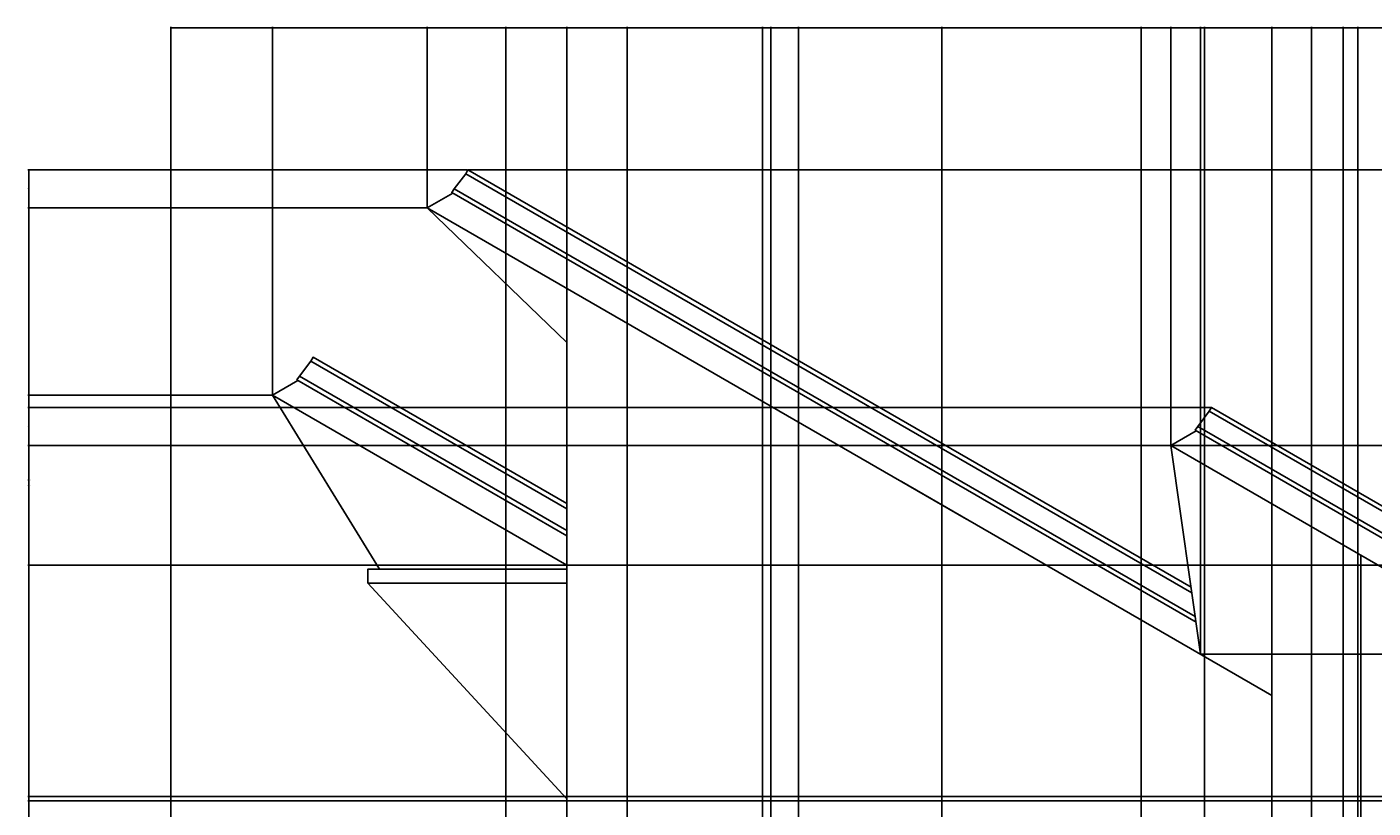
# Model space of a CAD drawing. Units: millimetres. Extents: x 171 to 1599, y 973 to 1509.
# Tile 4 of 7: x 951 to 1235, y 1343 to 1508. Entities that reach past the tile are written whole.
import ezdxf

# ---------------------------------------------------------------- set-up
doc = ezdxf.new("R2010")
doc.units = ezdxf.units.MM
doc.layers.add('A-ANNO-DIMS', color=2, linetype='Continuous', lineweight=18)
doc.layers.add('A-ELEV', color=7, linetype='Continuous', lineweight=25)
doc.styles.get("Standard").update_dxf_attribs({"font": 'arial.ttf'})
doc.dimstyles.get("Standard").update_dxf_attribs({"dimtxt": 0.18, "dimasz": 0.18, "dimexe": 0.18, "dimexo": 0.0625, "dimgap": 0.09, "dimtad": 0, "dimtih": 1, "dimtoh": 1, "dimdec": 1, "dimzin": 0, "dimdsep": 46, "dimlunit": 3, "dimtxsty": 'Standard', "dimcen": 0.09, "dimadec": 0, "dimazin": 0, "dimtfac": 1, "dimtdec": 1, "dimtofl": 0, "dimtmove": 0, "dimatfit": 3, "dimfxl": 1, "dimtolj": 1, "dimtzin": 0, "dimarcsym": 0})

# ---------------------------------------------------------------- blocks, each defined once
blk = doc.blocks.new('*D1')
at = {"layer": 'A-ANNO-DIMS', "color": 0, "lineweight": -2, "transparency": 16777216}
for p, q in [((980.93, 1194.55), (980.93, 1508.31)), ((981.11, 1508.13), (1274.61, 1508.13)), ((1568.85, 1508.13), (1275.36, 1508.13)), ((1569.03, 1215.31), (1569.03, 1508.31))]:
    blk.add_line(p, q, dxfattribs=at)
at = {"layer": 'A-ANNO-DIMS', "color": 0, "transparency": 16777216}
for points in [[(981.11, 1508.16), (981.11, 1508.1), (980.93, 1508.13)], [(1568.85, 1508.16), (1568.85, 1508.1), (1569.03, 1508.13)]]:
    blk.add_solid(points, dxfattribs=at)
at = {"layer": 'Defpoints', "color": 0, "transparency": 16777216}
for p in [(1569.03, 1508.13), (1569.03, 1215.25), (980.93, 1194.49)]:
    blk.add_point(p, dxfattribs=at)
at = {"layer": 'A-ANNO-DIMS', "color": 0, "transparency": 16777216, "insert": (1274.98, 1508.13), "char_height": 0.18, "attachment_point": 5}
blk.add_mtext('\\A1;588.1', dxfattribs=at)
blk = doc.blocks.new('*D2')
at = {"layer": 'A-ANNO-DIMS', "color": 0, "lineweight": -2, "transparency": 16777216}
for p, q in [((1043.70287, 1478.130098), (1599.212656, 1478.130098)), ((1599.032656, 1477.950098), (1599.032656, 1240.959874)), ((1599.032656, 1003.60965), (1599.032656, 1240.599874)), ((1348.449149, 1003.42965), (1599.212656, 1003.42965))]:
    blk.add_line(p, q, dxfattribs=at)
at = {"layer": 'A-ANNO-DIMS', "color": 0, "transparency": 16777216}
for points in [[(1599.002656, 1477.950098), (1599.062656, 1477.950098), (1599.032656, 1478.130098)], [(1599.002656, 1003.60965), (1599.062656, 1003.60965), (1599.032656, 1003.42965)]]:
    blk.add_solid(points, dxfattribs=at)
at = {"layer": 'Defpoints', "color": 0, "transparency": 16777216}
for p in [(1043.64037, 1478.130098), (1599.032656, 1478.130098), (1348.386649, 1003.42965)]:
    blk.add_point(p, dxfattribs=at)
at = {"layer": 'A-ANNO-DIMS', "color": 0, "transparency": 16777216, "insert": (1599.032656, 1240.779874), "char_height": 0.18, "attachment_point": 5}
blk.add_mtext('\\A1;474.7', dxfattribs=at)
blk = doc.blocks.new('*D17')
at = {"layer": 'A-ANNO-DIMS', "color": 0, "lineweight": -2, "transparency": 16777216}
for p, q in [((1105.76, 1344.87), (950.75, 1344.87)), ((950.93, 1344.69), (950.93, 1281.55)), ((950.93, 1218.05), (950.93, 1281.19)), ((1105.76, 1217.87), (950.75, 1217.87))]:
    blk.add_line(p, q, dxfattribs=at)
at = {"layer": 'A-ANNO-DIMS', "color": 0, "transparency": 16777216}
for points in [[(950.9, 1344.69), (950.96, 1344.69), (950.93, 1344.87)], [(950.9, 1218.05), (950.96, 1218.05), (950.93, 1217.87)]]:
    blk.add_solid(points, dxfattribs=at)
at = {"layer": 'Defpoints', "color": 0, "transparency": 16777216}
for p in [(950.93, 1344.87), (1105.82, 1344.87), (1105.82, 1217.87)]:
    blk.add_point(p, dxfattribs=at)
at = {"layer": 'A-ANNO-DIMS', "color": 0, "transparency": 16777216, "insert": (950.93, 1281.37), "char_height": 0.18, "attachment_point": 5}
blk.add_mtext('\\A1;127', dxfattribs=at)
blk = doc.blocks.new('*D18')
at = {"layer": 'A-ANNO-DIMS', "color": 0, "lineweight": -2, "transparency": 16777216}
for p, q in [((1043.58, 1478.13), (950.75, 1478.13)), ((950.93, 1477.95), (950.93, 1411.68)), ((950.93, 1345.05), (950.93, 1411.32)), ((1105.76, 1344.87), (950.75, 1344.87))]:
    blk.add_line(p, q, dxfattribs=at)
at = {"layer": 'A-ANNO-DIMS', "color": 0, "transparency": 16777216}
for points in [[(950.9, 1477.95), (950.96, 1477.95), (950.93, 1478.13)], [(950.9, 1345.05), (950.96, 1345.05), (950.93, 1344.87)]]:
    blk.add_solid(points, dxfattribs=at)
at = {"layer": 'Defpoints', "color": 0, "transparency": 16777216}
for p in [(950.93, 1478.13), (1043.64, 1478.13), (1105.82, 1344.87)]:
    blk.add_point(p, dxfattribs=at)
at = {"layer": 'A-ANNO-DIMS', "color": 0, "transparency": 16777216, "insert": (950.93, 1411.5), "char_height": 0.18, "attachment_point": 5}
blk.add_mtext('\\A1;133.26', dxfattribs=at)
blk = doc.blocks.new('*D38')
at = {"layer": 'A-ANNO-DIMS', "color": 0, "lineweight": -2, "transparency": 16777216}
for p, q in [((980.93, 1203.86), (980.93, 1508.31)), ((981.11, 1508.13), (991.19, 1508.13)), ((1002.21, 1508.13), (992.12, 1508.13)), ((1002.39, 1430.6), (1002.39, 1508.31))]:
    blk.add_line(p, q, dxfattribs=at)
at = {"layer": 'A-ANNO-DIMS', "color": 0, "transparency": 16777216}
for points in [[(981.11, 1508.16), (981.11, 1508.1), (980.93, 1508.13)], [(1002.21, 1508.16), (1002.21, 1508.1), (1002.39, 1508.13)]]:
    blk.add_solid(points, dxfattribs=at)
at = {"layer": 'Defpoints', "color": 0, "transparency": 16777216}
for p in [(1002.39, 1508.13), (1002.39, 1430.53), (980.93, 1203.79)]:
    blk.add_point(p, dxfattribs=at)
at = {"layer": 'A-ANNO-DIMS', "color": 0, "transparency": 16777216, "insert": (991.66, 1508.13), "char_height": 0.18, "attachment_point": 5}
blk.add_mtext('\\A1;21.455', dxfattribs=at)
blk = doc.blocks.new('*D39')
at = {"layer": 'A-ANNO-DIMS', "color": 0, "lineweight": -2, "transparency": 16777216}
for p, q in [((1002.39, 1430.6), (1002.39, 1508.31)), ((1002.57, 1508.13), (1033.05, 1508.13)), ((1064.32, 1508.13), (1033.84, 1508.13)), ((1064.5, 1394.73), (1064.5, 1508.31))]:
    blk.add_line(p, q, dxfattribs=at)
at = {"layer": 'A-ANNO-DIMS', "color": 0, "transparency": 16777216}
for points in [[(1002.57, 1508.16), (1002.57, 1508.1), (1002.39, 1508.13)], [(1064.32, 1508.16), (1064.32, 1508.1), (1064.5, 1508.13)]]:
    blk.add_solid(points, dxfattribs=at)
at = {"layer": 'Defpoints', "color": 0, "transparency": 16777216}
for p in [(1064.5, 1508.13), (1002.39, 1430.53), (1064.5, 1394.67)]:
    blk.add_point(p, dxfattribs=at)
at = {"layer": 'A-ANNO-DIMS', "color": 0, "transparency": 16777216, "insert": (1033.45, 1508.13), "char_height": 0.18, "attachment_point": 5}
blk.add_mtext('\\A1;62.12', dxfattribs=at)
blk = doc.blocks.new('*D40')
at = {"layer": 'A-ANNO-DIMS', "color": 0, "lineweight": -2, "transparency": 16777216}
for p, q in [((1002.39, 1430.6), (1002.39, 1508.31)), ((1002.57, 1508.13), (1018.33, 1508.13)), ((1034.88, 1508.13), (1019.12, 1508.13)), ((1035.06, 1470.15), (1035.06, 1508.31))]:
    blk.add_line(p, q, dxfattribs=at)
at = {"layer": 'A-ANNO-DIMS', "color": 0, "transparency": 16777216}
for points in [[(1002.57, 1508.16), (1002.57, 1508.1), (1002.39, 1508.13)], [(1034.88, 1508.16), (1034.88, 1508.1), (1035.06, 1508.13)]]:
    blk.add_solid(points, dxfattribs=at)
at = {"layer": 'Defpoints', "color": 0, "transparency": 16777216}
for p in [(1035.06, 1508.13), (1035.06, 1470.09), (1002.39, 1430.53)]:
    blk.add_point(p, dxfattribs=at)
at = {"layer": 'A-ANNO-DIMS', "color": 0, "transparency": 16777216, "insert": (1018.72, 1508.13), "char_height": 0.18, "attachment_point": 5}
blk.add_mtext('\\A1;32.68', dxfattribs=at)
blk = doc.blocks.new('*D41')
at = {"layer": 'A-ANNO-DIMS', "color": 0, "lineweight": -2, "transparency": 16777216}
for p, q in [((1035.06, 1470.15), (1035.06, 1508.31)), ((1035.24, 1508.13), (1116.22, 1508.13)), ((1198.11, 1508.13), (1117.13, 1508.13)), ((1198.29, 1375.91), (1198.29, 1508.31))]:
    blk.add_line(p, q, dxfattribs=at)
at = {"layer": 'A-ANNO-DIMS', "color": 0, "transparency": 16777216}
for points in [[(1035.24, 1508.16), (1035.24, 1508.1), (1035.06, 1508.13)], [(1198.11, 1508.16), (1198.11, 1508.1), (1198.29, 1508.13)]]:
    blk.add_solid(points, dxfattribs=at)
at = {"layer": 'Defpoints', "color": 0, "transparency": 16777216}
for p in [(1198.29, 1508.13), (1035.06, 1470.09), (1198.29, 1375.85)]:
    blk.add_point(p, dxfattribs=at)
at = {"layer": 'A-ANNO-DIMS', "color": 0, "transparency": 16777216, "insert": (1116.68, 1508.13), "char_height": 0.18, "attachment_point": 5}
blk.add_mtext('\\A1;163.23', dxfattribs=at)
blk = doc.blocks.new('*D42')
at = {"layer": 'A-ANNO-DIMS', "color": 0, "lineweight": -2, "transparency": 16777216}
for p, q in [((1192.02, 1419.99), (1192.02, 1508.31)), ((1192.2, 1508.13), (1378.72, 1508.13)), ((1566.18, 1508.13), (1379.65, 1508.13)), ((1566.36, 1203.87), (1566.36, 1508.31))]:
    blk.add_line(p, q, dxfattribs=at)
at = {"layer": 'A-ANNO-DIMS', "color": 0, "transparency": 16777216}
for points in [[(1192.2, 1508.16), (1192.2, 1508.1), (1192.02, 1508.13)], [(1566.18, 1508.16), (1566.18, 1508.1), (1566.36, 1508.13)]]:
    blk.add_solid(points, dxfattribs=at)
at = {"layer": 'Defpoints', "color": 0, "transparency": 16777216}
for p in [(1566.36, 1508.13), (1192.02, 1419.93), (1566.36, 1203.8)]:
    blk.add_point(p, dxfattribs=at)
at = {"layer": 'A-ANNO-DIMS', "color": 0, "transparency": 16777216, "insert": (1379.19, 1508.13), "char_height": 0.18, "attachment_point": 5}
blk.add_mtext('\\A1;374.34', dxfattribs=at)
blk = doc.blocks.new('*D43')
at = {"layer": 'A-ANNO-DIMS', "color": 0, "lineweight": -2, "transparency": 16777216}
for p, q in [((1002.32, 1430.53), (950.75, 1430.53)), ((950.93, 1430.35), (950.93, 1412.78)), ((950.93, 1394.85), (950.93, 1412.42)), ((1064.44, 1394.67), (950.75, 1394.67))]:
    blk.add_line(p, q, dxfattribs=at)
at = {"layer": 'A-ANNO-DIMS', "color": 0, "transparency": 16777216}
for points in [[(950.9, 1430.35), (950.96, 1430.35), (950.93, 1430.53)], [(950.9, 1394.85), (950.96, 1394.85), (950.93, 1394.67)]]:
    blk.add_solid(points, dxfattribs=at)
at = {"layer": 'Defpoints', "color": 0, "transparency": 16777216}
for p in [(1002.39, 1430.53), (950.93, 1394.67), (1064.5, 1394.67)]:
    blk.add_point(p, dxfattribs=at)
at = {"layer": 'A-ANNO-DIMS', "color": 0, "transparency": 16777216, "insert": (950.93, 1412.6), "char_height": 0.18, "attachment_point": 5}
blk.add_mtext('\\A1;35.865', dxfattribs=at)
blk = doc.blocks.new('*D44')
at = {"layer": 'A-ANNO-DIMS', "color": 0, "lineweight": -2, "transparency": 16777216}
for p, q in [((1043.58, 1478.13), (950.75, 1478.13)), ((950.93, 1477.95), (950.93, 1474.29)), ((950.93, 1470.27), (950.93, 1473.93)), ((1035, 1470.09), (950.75, 1470.09))]:
    blk.add_line(p, q, dxfattribs=at)
at = {"layer": 'A-ANNO-DIMS', "color": 0, "transparency": 16777216}
for points in [[(950.9, 1477.95), (950.96, 1477.95), (950.93, 1478.13)], [(950.9, 1470.27), (950.96, 1470.27), (950.93, 1470.09)]]:
    blk.add_solid(points, dxfattribs=at)
at = {"layer": 'Defpoints', "color": 0, "transparency": 16777216}
for p in [(950.93, 1478.13), (1043.64, 1478.13), (1035.06, 1470.09)]:
    blk.add_point(p, dxfattribs=at)
at = {"layer": 'A-ANNO-DIMS', "color": 0, "transparency": 16777216, "insert": (950.93, 1474.11), "char_height": 0.18, "attachment_point": 5}
blk.add_mtext('\\A1;8.04', dxfattribs=at)
blk = doc.blocks.new('*D45')
at = {"layer": 'A-ANNO-DIMS', "color": 0, "lineweight": -2, "transparency": 16777216}
for p, q in [((1064.57, 1394.67), (1599.21, 1394.67)), ((1599.03, 1394.49), (1599.03, 1369.95)), ((1599.03, 1345.05), (1599.03, 1369.59)), ((1105.88, 1344.87), (1599.21, 1344.87))]:
    blk.add_line(p, q, dxfattribs=at)
at = {"layer": 'A-ANNO-DIMS', "color": 0, "transparency": 16777216}
for points in [[(1599, 1394.49), (1599.06, 1394.49), (1599.03, 1394.67)], [(1599, 1345.05), (1599.06, 1345.05), (1599.03, 1344.87)]]:
    blk.add_solid(points, dxfattribs=at)
at = {"layer": 'Defpoints', "color": 0, "transparency": 16777216}
for p in [(1064.5, 1394.67), (1105.82, 1344.87), (1599.03, 1344.87)]:
    blk.add_point(p, dxfattribs=at)
at = {"layer": 'A-ANNO-DIMS', "color": 0, "transparency": 16777216, "insert": (1599.03, 1369.77), "char_height": 0.18, "attachment_point": 5}
blk.add_mtext('\\A1;49.80', dxfattribs=at)
blk = doc.blocks.new('*D46')
at = {"layer": 'A-ANNO-DIMS', "color": 0, "lineweight": -2, "transparency": 16777216}
for p, q in [((1198.36, 1375.85), (1599.21, 1375.85)), ((1599.03, 1375.67), (1599.03, 1360.54)), ((1599.03, 1345.05), (1599.03, 1360.18)), ((1185.8, 1344.87), (1599.21, 1344.87))]:
    blk.add_line(p, q, dxfattribs=at)
at = {"layer": 'A-ANNO-DIMS', "color": 0, "transparency": 16777216}
for points in [[(1599, 1375.67), (1599.06, 1375.67), (1599.03, 1375.85)], [(1599, 1345.05), (1599.06, 1345.05), (1599.03, 1344.87)]]:
    blk.add_solid(points, dxfattribs=at)
at = {"layer": 'Defpoints', "color": 0, "transparency": 16777216}
for p in [(1198.29, 1375.85), (1599.03, 1375.85), (1185.73, 1344.87)]:
    blk.add_point(p, dxfattribs=at)
at = {"layer": 'A-ANNO-DIMS', "color": 0, "transparency": 16777216, "insert": (1599.03, 1360.36), "char_height": 0.18, "attachment_point": 5}
blk.add_mtext('\\A1;30.976', dxfattribs=at)
blk = doc.blocks.new('*D47')
at = {"layer": 'A-ANNO-DIMS', "color": 0, "lineweight": -2, "transparency": 16777216}
for p, q in [((1192.08, 1419.93), (1599.21, 1419.93)), ((1599.03, 1419.75), (1599.03, 1312.05)), ((1599.03, 1203.98), (1599.03, 1311.68)), ((1566.42, 1203.8), (1599.21, 1203.8))]:
    blk.add_line(p, q, dxfattribs=at)
at = {"layer": 'A-ANNO-DIMS', "color": 0, "transparency": 16777216}
for points in [[(1599, 1419.75), (1599.06, 1419.75), (1599.03, 1419.93)], [(1599, 1203.98), (1599.06, 1203.98), (1599.03, 1203.8)]]:
    blk.add_solid(points, dxfattribs=at)
at = {"layer": 'Defpoints', "color": 0, "transparency": 16777216}
for p in [(1192.02, 1419.93), (1566.36, 1203.8), (1599.03, 1203.8)]:
    blk.add_point(p, dxfattribs=at)
at = {"layer": 'A-ANNO-DIMS', "color": 0, "transparency": 16777216, "insert": (1599.03, 1311.87), "char_height": 0.18, "attachment_point": 5}
blk.add_mtext('\\A1;216.13', dxfattribs=at)
blk = doc.blocks.new('*D48')
at = {"layer": 'A-ANNO-DIMS', "color": 0, "lineweight": -2, "transparency": 16777216}
for p, q in [((1200.53, 1427.97), (950.75, 1427.97)), ((950.93, 1427.79), (950.93, 1424.13)), ((950.93, 1420.11), (950.93, 1423.77)), ((1191.95, 1419.93), (950.75, 1419.93))]:
    blk.add_line(p, q, dxfattribs=at)
at = {"layer": 'A-ANNO-DIMS', "color": 0, "transparency": 16777216}
for points in [[(950.9, 1427.79), (950.96, 1427.79), (950.93, 1427.97)], [(950.9, 1420.11), (950.96, 1420.11), (950.93, 1419.93)]]:
    blk.add_solid(points, dxfattribs=at)
at = {"layer": 'Defpoints', "color": 0, "transparency": 16777216}
for p in [(950.93, 1427.97), (1200.59, 1427.97), (1192.02, 1419.93)]:
    blk.add_point(p, dxfattribs=at)
at = {"layer": 'A-ANNO-DIMS', "color": 0, "transparency": 16777216, "insert": (950.93, 1423.95), "char_height": 0.18, "attachment_point": 5}
blk.add_mtext('\\A1;8.04', dxfattribs=at)
blk = doc.blocks.new('*D49')
at = {"layer": 'A-ANNO-DIMS', "color": 0, "lineweight": -2, "transparency": 16777216}
for p, q in [((1064.5, 1203.86), (1064.5, 1508.31)), ((1064.68, 1508.13), (1084.78, 1508.13)), ((1105.64, 1508.13), (1085.54, 1508.13)), ((1105.82, 1344.93), (1105.82, 1508.31))]:
    blk.add_line(p, q, dxfattribs=at)
at = {"layer": 'A-ANNO-DIMS', "color": 0, "transparency": 16777216}
for points in [[(1064.68, 1508.16), (1064.68, 1508.1), (1064.5, 1508.13)], [(1105.64, 1508.16), (1105.64, 1508.1), (1105.82, 1508.13)]]:
    blk.add_solid(points, dxfattribs=at)
at = {"layer": 'Defpoints', "color": 0, "transparency": 16777216}
for p in [(1105.82, 1508.13), (1105.82, 1344.87), (1064.5, 1203.79)]:
    blk.add_point(p, dxfattribs=at)
at = {"layer": 'A-ANNO-DIMS', "color": 0, "transparency": 16777216, "insert": (1085.16, 1508.13), "char_height": 0.18, "attachment_point": 5}
blk.add_mtext('\\A1;41.31', dxfattribs=at)
blk = doc.blocks.new('*D50')
at = {"layer": 'A-ANNO-DIMS', "color": 0, "lineweight": -2, "transparency": 16777216}
for p, q in [((1105.82, 1344.93), (1105.82, 1508.31)), ((1106, 1508.13), (1145.38, 1508.13)), ((1185.55, 1508.13), (1146.17, 1508.13)), ((1185.73, 1344.93), (1185.73, 1508.31))]:
    blk.add_line(p, q, dxfattribs=at)
at = {"layer": 'A-ANNO-DIMS', "color": 0, "transparency": 16777216}
for points in [[(1106, 1508.16), (1106, 1508.1), (1105.82, 1508.13)], [(1185.55, 1508.16), (1185.55, 1508.1), (1185.73, 1508.13)]]:
    blk.add_solid(points, dxfattribs=at)
at = {"layer": 'Defpoints', "color": 0, "transparency": 16777216}
for p in [(1185.73, 1508.13), (1105.82, 1344.87), (1185.73, 1344.87)]:
    blk.add_point(p, dxfattribs=at)
at = {"layer": 'A-ANNO-DIMS', "color": 0, "transparency": 16777216, "insert": (1145.78, 1508.13), "char_height": 0.18, "attachment_point": 5}
blk.add_mtext('\\A1;79.92', dxfattribs=at)
blk = doc.blocks.new('*D51')
at = {"layer": 'A-ANNO-DIMS', "color": 0, "lineweight": -2, "transparency": 16777216}
for p, q in [((1185.73, 1344.93), (1185.73, 1508.31)), ((1185.91, 1508.13), (1199.08, 1508.13)), ((1213.17, 1508.13), (1200.01, 1508.13)), ((1213.35, 1203.86), (1213.35, 1508.31))]:
    blk.add_line(p, q, dxfattribs=at)
at = {"layer": 'A-ANNO-DIMS', "color": 0, "transparency": 16777216}
for points in [[(1185.91, 1508.16), (1185.91, 1508.1), (1185.73, 1508.13)], [(1213.17, 1508.16), (1213.17, 1508.1), (1213.35, 1508.13)]]:
    blk.add_solid(points, dxfattribs=at)
at = {"layer": 'Defpoints', "color": 0, "transparency": 16777216}
for p in [(1213.35, 1508.13), (1185.73, 1344.87), (1213.35, 1203.79)]:
    blk.add_point(p, dxfattribs=at)
at = {"layer": 'A-ANNO-DIMS', "color": 0, "transparency": 16777216, "insert": (1199.54, 1508.13), "char_height": 0.18, "attachment_point": 5}
blk.add_mtext('\\A1;27.614', dxfattribs=at)
blk = doc.blocks.new('*D61')
at = {"layer": 'A-ANNO-DIMS', "color": 0, "lineweight": -2, "transparency": 16777216}
for p, q in [((1320.26, 1345.85), (950.75, 1345.85)), ((950.93, 1345.67), (950.93, 1269.24)), ((950.93, 1192.45), (950.93, 1268.88)), ((1320.26, 1192.27), (950.75, 1192.27))]:
    blk.add_line(p, q, dxfattribs=at)
at = {"layer": 'A-ANNO-DIMS', "color": 0, "transparency": 16777216}
for points in [[(950.9, 1345.67), (950.96, 1345.67), (950.93, 1345.85)], [(950.9, 1192.45), (950.96, 1192.45), (950.93, 1192.27)]]:
    blk.add_solid(points, dxfattribs=at)
at = {"layer": 'Defpoints', "color": 0, "transparency": 16777216}
for p in [(950.93, 1345.85), (1320.32, 1345.85), (1320.32, 1192.27)]:
    blk.add_point(p, dxfattribs=at)
at = {"layer": 'A-ANNO-DIMS', "color": 0, "transparency": 16777216, "insert": (950.93, 1269.06), "char_height": 0.18, "attachment_point": 5}
blk.add_mtext('\\A1;153.59', dxfattribs=at)
blk = doc.blocks.new('*D64')
at = {"layer": 'A-ANNO-DIMS', "color": 0, "lineweight": -2, "transparency": 16777216}
for p, q in [((1051.62, 1177.93), (1051.62, 1508.31)), ((1051.8, 1508.13), (1057.61, 1508.13)), ((1064.32, 1508.13), (1058.52, 1508.13)), ((1064.5, 1177.93), (1064.5, 1508.31))]:
    blk.add_line(p, q, dxfattribs=at)
at = {"layer": 'A-ANNO-DIMS', "color": 0, "transparency": 16777216}
for points in [[(1051.8, 1508.16), (1051.8, 1508.1), (1051.62, 1508.13)], [(1064.32, 1508.16), (1064.32, 1508.1), (1064.5, 1508.13)]]:
    blk.add_solid(points, dxfattribs=at)
at = {"layer": 'Defpoints', "color": 0, "transparency": 16777216}
for p in [(1064.5, 1508.13), (1051.62, 1177.87), (1064.5, 1177.87)]:
    blk.add_point(p, dxfattribs=at)
at = {"layer": 'A-ANNO-DIMS', "color": 0, "transparency": 16777216, "insert": (1058.06, 1508.13), "char_height": 0.18, "attachment_point": 5}
blk.add_mtext('\\A1;12.882', dxfattribs=at)
blk = doc.blocks.new('*D65')
at = {"layer": 'A-ANNO-DIMS', "color": 0, "lineweight": -2, "transparency": 16777216}
for p, q in [((1064.5, 1177.93), (1064.5, 1508.31)), ((1064.68, 1508.13), (1070.43, 1508.13)), ((1077.09, 1508.13), (1071.34, 1508.13)), ((1077.27, 1177.93), (1077.27, 1508.31))]:
    blk.add_line(p, q, dxfattribs=at)
at = {"layer": 'A-ANNO-DIMS', "color": 0, "transparency": 16777216}
for points in [[(1064.68, 1508.16), (1064.68, 1508.1), (1064.5, 1508.13)], [(1077.09, 1508.16), (1077.09, 1508.1), (1077.27, 1508.13)]]:
    blk.add_solid(points, dxfattribs=at)
at = {"layer": 'Defpoints', "color": 0, "transparency": 16777216}
for p in [(1077.27, 1508.13), (1064.5, 1177.87), (1077.27, 1177.87)]:
    blk.add_point(p, dxfattribs=at)
at = {"layer": 'A-ANNO-DIMS', "color": 0, "transparency": 16777216, "insert": (1070.89, 1508.13), "char_height": 0.18, "attachment_point": 5}
blk.add_mtext('\\A1;12.767', dxfattribs=at)
blk = doc.blocks.new('*D66')
at = {"layer": 'A-ANNO-DIMS', "color": 0, "lineweight": -2, "transparency": 16777216}
for p, q in [((1077.27, 1177.93), (1077.27, 1508.31)), ((1077.45, 1508.13), (1092.02, 1508.13)), ((1107.38, 1508.13), (1092.81, 1508.13)), ((1107.56, 1177.93), (1107.56, 1508.31))]:
    blk.add_line(p, q, dxfattribs=at)
at = {"layer": 'A-ANNO-DIMS', "color": 0, "transparency": 16777216}
for points in [[(1077.45, 1508.16), (1077.45, 1508.1), (1077.27, 1508.13)], [(1107.38, 1508.16), (1107.38, 1508.1), (1107.56, 1508.13)]]:
    blk.add_solid(points, dxfattribs=at)
at = {"layer": 'Defpoints', "color": 0, "transparency": 16777216}
for p in [(1107.56, 1508.13), (1077.27, 1177.87), (1107.56, 1177.87)]:
    blk.add_point(p, dxfattribs=at)
at = {"layer": 'A-ANNO-DIMS', "color": 0, "transparency": 16777216, "insert": (1092.42, 1508.13), "char_height": 0.18, "attachment_point": 5}
blk.add_mtext('\\A1;30.29', dxfattribs=at)
blk = doc.blocks.new('*D67')
at = {"layer": 'A-ANNO-DIMS', "color": 0, "lineweight": -2, "transparency": 16777216}
for p, q in [((1107.56, 1177.93), (1107.56, 1508.31)), ((1107.74, 1508.13), (1110.09, 1508.13)), ((1113.23, 1508.13), (1110.88, 1508.13)), ((1113.41, 1177.93), (1113.41, 1508.31))]:
    blk.add_line(p, q, dxfattribs=at)
at = {"layer": 'A-ANNO-DIMS', "color": 0, "transparency": 16777216}
for points in [[(1107.74, 1508.16), (1107.74, 1508.1), (1107.56, 1508.13)], [(1113.23, 1508.16), (1113.23, 1508.1), (1113.41, 1508.13)]]:
    blk.add_solid(points, dxfattribs=at)
at = {"layer": 'Defpoints', "color": 0, "transparency": 16777216}
for p in [(1113.41, 1508.13), (1107.56, 1177.87), (1113.41, 1177.87)]:
    blk.add_point(p, dxfattribs=at)
at = {"layer": 'A-ANNO-DIMS', "color": 0, "transparency": 16777216, "insert": (1110.49, 1508.13), "char_height": 0.18, "attachment_point": 5}
blk.add_mtext('\\A1;5.847', dxfattribs=at)
blk = doc.blocks.new('*D68')
at = {"layer": 'A-ANNO-DIMS', "color": 0, "lineweight": -2, "transparency": 16777216}
for p, q in [((1113.41, 1177.93), (1113.41, 1508.31)), ((1113.59, 1508.13), (1128.16, 1508.13)), ((1143.52, 1508.13), (1128.95, 1508.13)), ((1143.7, 1177.93), (1143.7, 1508.31))]:
    blk.add_line(p, q, dxfattribs=at)
at = {"layer": 'A-ANNO-DIMS', "color": 0, "transparency": 16777216}
for points in [[(1113.59, 1508.16), (1113.59, 1508.1), (1113.41, 1508.13)], [(1143.52, 1508.16), (1143.52, 1508.1), (1143.7, 1508.13)]]:
    blk.add_solid(points, dxfattribs=at)
at = {"layer": 'Defpoints', "color": 0, "transparency": 16777216}
for p in [(1143.7, 1508.13), (1113.41, 1177.87), (1143.7, 1177.87)]:
    blk.add_point(p, dxfattribs=at)
at = {"layer": 'A-ANNO-DIMS', "color": 0, "transparency": 16777216, "insert": (1128.55, 1508.13), "char_height": 0.18, "attachment_point": 5}
blk.add_mtext('\\A1;30.29', dxfattribs=at)
blk = doc.blocks.new('*D69')
at = {"layer": 'A-ANNO-DIMS', "color": 0, "lineweight": -2, "transparency": 16777216}
for p, q in [((1143.7, 1177.93), (1143.7, 1508.31)), ((1143.88, 1508.13), (1171.03, 1508.13)), ((1198.93, 1508.13), (1171.78, 1508.13)), ((1199.11, 1177.93), (1199.11, 1508.31))]:
    blk.add_line(p, q, dxfattribs=at)
at = {"layer": 'A-ANNO-DIMS', "color": 0, "transparency": 16777216}
for points in [[(1143.88, 1508.16), (1143.88, 1508.1), (1143.7, 1508.13)], [(1198.93, 1508.16), (1198.93, 1508.1), (1199.11, 1508.13)]]:
    blk.add_solid(points, dxfattribs=at)
at = {"layer": 'Defpoints', "color": 0, "transparency": 16777216}
for p in [(1199.11, 1508.13), (1143.7, 1177.87), (1199.11, 1177.87)]:
    blk.add_point(p, dxfattribs=at)
at = {"layer": 'A-ANNO-DIMS', "color": 0, "transparency": 16777216, "insert": (1171.4, 1508.13), "char_height": 0.18, "attachment_point": 5}
blk.add_mtext('\\A1;55.41', dxfattribs=at)
blk = doc.blocks.new('*D70')
at = {"layer": 'A-ANNO-DIMS', "color": 0, "lineweight": -2, "transparency": 16777216}
for p, q in [((1199.11, 1177.93), (1199.11, 1508.31)), ((1199.29, 1508.13), (1210.04, 1508.13)), ((1221.54, 1508.13), (1210.79, 1508.13)), ((1221.72, 1177.93), (1221.72, 1508.31))]:
    blk.add_line(p, q, dxfattribs=at)
at = {"layer": 'A-ANNO-DIMS', "color": 0, "transparency": 16777216}
for points in [[(1199.29, 1508.16), (1199.29, 1508.1), (1199.11, 1508.13)], [(1221.54, 1508.16), (1221.54, 1508.1), (1221.72, 1508.13)]]:
    blk.add_solid(points, dxfattribs=at)
at = {"layer": 'Defpoints', "color": 0, "transparency": 16777216}
for p in [(1221.72, 1508.13), (1199.11, 1177.87), (1221.72, 1177.87)]:
    blk.add_point(p, dxfattribs=at)
at = {"layer": 'A-ANNO-DIMS', "color": 0, "transparency": 16777216, "insert": (1210.41, 1508.13), "char_height": 0.18, "attachment_point": 5}
blk.add_mtext('\\A1;22.61', dxfattribs=at)
blk = doc.blocks.new('*D71')
at = {"layer": 'A-ANNO-DIMS', "color": 0, "lineweight": -2, "transparency": 16777216}
for p, q in [((1221.72, 1177.93), (1221.72, 1508.31)), ((1221.9, 1508.13), (1224.73, 1508.13)), ((1228.22, 1508.13), (1225.38, 1508.13)), ((1228.4, 1114.32), (1228.4, 1508.31))]:
    blk.add_line(p, q, dxfattribs=at)
at = {"layer": 'A-ANNO-DIMS', "color": 0, "transparency": 16777216}
for points in [[(1221.9, 1508.16), (1221.9, 1508.1), (1221.72, 1508.13)], [(1228.22, 1508.16), (1228.22, 1508.1), (1228.4, 1508.13)]]:
    blk.add_solid(points, dxfattribs=at)
at = {"layer": 'Defpoints', "color": 0, "transparency": 16777216}
for p in [(1228.4, 1508.13), (1221.72, 1177.87), (1228.4, 1114.25)]:
    blk.add_point(p, dxfattribs=at)
at = {"layer": 'A-ANNO-DIMS', "color": 0, "transparency": 16777216, "insert": (1225.06, 1508.13), "char_height": 0.18, "attachment_point": 5}
blk.add_mtext('\\A1;6.68', dxfattribs=at)
blk = doc.blocks.new('*D72')
at = {"layer": 'A-ANNO-DIMS', "color": 0, "lineweight": -2, "transparency": 16777216}
for p, q in [((1228.4, 1114.32), (1228.4, 1508.31)), ((1228.58, 1508.13), (1229.61, 1508.13)), ((1231.28, 1508.13), (1230.25, 1508.13)), ((1231.46, 1114.32), (1231.46, 1508.31))]:
    blk.add_line(p, q, dxfattribs=at)
at = {"layer": 'A-ANNO-DIMS', "color": 0, "transparency": 16777216}
for points in [[(1228.58, 1508.16), (1228.58, 1508.1), (1228.4, 1508.13)], [(1231.28, 1508.16), (1231.28, 1508.1), (1231.46, 1508.13)]]:
    blk.add_solid(points, dxfattribs=at)
at = {"layer": 'Defpoints', "color": 0, "transparency": 16777216}
for p in [(1231.46, 1508.13), (1228.4, 1114.25), (1231.46, 1114.25)]:
    blk.add_point(p, dxfattribs=at)
at = {"layer": 'A-ANNO-DIMS', "color": 0, "transparency": 16777216, "insert": (1229.93, 1508.13), "char_height": 0.18, "attachment_point": 5}
blk.add_mtext('\\A1;3.06', dxfattribs=at)
blk = doc.blocks.new('*D73')
at = {"layer": 'A-ANNO-DIMS', "color": 0, "lineweight": -2, "transparency": 16777216}
for p, q in [((1231.46, 1114.32), (1231.46, 1508.31)), ((1231.64, 1508.13), (1234.06, 1508.13)), ((1237.13, 1508.13), (1234.71, 1508.13)), ((1237.31, 1162.35), (1237.31, 1508.31))]:
    blk.add_line(p, q, dxfattribs=at)
at = {"layer": 'A-ANNO-DIMS', "color": 0, "transparency": 16777216}
for points in [[(1231.64, 1508.16), (1231.64, 1508.1), (1231.46, 1508.13)], [(1237.13, 1508.16), (1237.13, 1508.1), (1237.31, 1508.13)]]:
    blk.add_solid(points, dxfattribs=at)
at = {"layer": 'Defpoints', "color": 0, "transparency": 16777216}
for p in [(1237.31, 1508.13), (1237.31, 1162.29), (1231.46, 1114.25)]:
    blk.add_point(p, dxfattribs=at)
at = {"layer": 'A-ANNO-DIMS', "color": 0, "transparency": 16777216, "insert": (1234.38, 1508.13), "char_height": 0.18, "attachment_point": 5}
blk.add_mtext('\\A1;5.85', dxfattribs=at)

msp = doc.modelspace()

# ---------------------------------------------------------------- linework, layer by layer
at = {"layer": 'A-ELEV'}
for p, q in [((1043.1682, 1477.3124), (1196.447, 1388.8168)), ((1040.7486, 1474.1058), (1197.1614, 1383.8008)), ((1148.9051, 1404.3628), (1035.0626, 1470.0898)), ((1064.505, 1203.7941), (1064.505, 1453.0912)), ((1010.4912, 1437.7559), (1064.505, 1406.5711)), ((1007.5452, 1433.7629), (1064.505, 1400.8772)), ((1064.505, 1394.6687), (1002.3855, 1430.5334)), ((1197.176, 1423.1592), (1197.7023, 1423.9457)), ((1192.0162, 1419.9297), (1198.2939, 1375.8481)), ((1135.1656, 1412.2952), (1213.3488, 1367.1562)), ((1213.3488, 1203.7941), (1213.3488, 1407.6133)), ((1022.4961, 1390.8634), (1064.505, 1345.3593))]:
    msp.add_line(p, q, dxfattribs=at)
for points in [[(1040.2223, 1473.3193), (1040.7486, 1474.1058), (1043.1682, 1477.3124), (1043.6404, 1478.1301), (1196.2778, 1390.0048)], [(1197.3305, 1382.6128), (1040.2223, 1473.3193), (1040.4393, 1473.194), (1035.0626, 1470.0898), (1064.505, 1441.6631)], [(1008.0715, 1434.5494), (1010.4912, 1437.7559), (1010.9633, 1438.5737), (1064.505, 1407.6614)], [(1064.505, 1401.9675), (1008.0715, 1434.5494), (1007.5452, 1433.7629), (1007.7622, 1433.6376), (1002.3855, 1430.5334), (1024.973, 1393.7984)], [(1200.1219, 1427.1523), (1200.594, 1427.97), (1569.0327, 1215.2519), (1568.5605, 1214.4341), (1566.9934, 1210.7354), (1566.5754, 1209.8864), (1197.176, 1423.1592), (1197.3929, 1423.034), (1192.0162, 1419.9297), (1305.8587, 1354.2027), (1566.3585, 1203.8031), (1566.3585, 1210.0116)], [(1566.9934, 1210.7354), (1197.7023, 1423.9457), (1200.1219, 1427.1523), (1568.5605, 1214.4341)], [(1232.0993, 1203.7941), (1232.0993, 1396.7877)]]:
    msp.add_lwpolyline(points, dxfattribs=at)
for points in [[(1064.505, 1390.8634), (1022.4961, 1390.8634), (1022.4961, 1393.7984), (1064.505, 1393.7984)], [(1185.7346, 1217.867), (1105.8176, 1217.867), (1105.8176, 1344.8717), (1185.7346, 1344.8717)]]:
    msp.add_lwpolyline(points, close=True, dxfattribs=at)

# ---------------------------------------------------------------- dimensions: what is measured, and where the dimension line sits
at = {"layer": 'A-ANNO-DIMS'}
for base, p1, p2, override, picture, middle in [((1569.0327, 1508.1301), (980.9303, 1194.488), (1569.0327, 1215.2519), {"dimdec": 1, "dimlfac": 1, "dimrnd": 0, "dimzin": 0, "dimdsep": 46, "dimlunit": 2}, '*D1', (1274.9815, 1508.1301)), ((1002.3855, 1508.1301), (980.9303, 1203.7941), (1002.3855, 1430.5334), {"dimdec": 3, "dimlfac": 1, "dimrnd": 0, "dimzin": 0, "dimdsep": 46, "dimlunit": 2}, '*D38', (991.6579, 1508.1301)), ((1064.505, 1508.1301), (1002.3855, 1430.5334), (1064.505, 1394.6687), {"dimdec": 2, "dimlfac": 1, "dimrnd": 0, "dimzin": 0, "dimdsep": 46, "dimlunit": 2}, '*D39', (1033.4452, 1508.1301)), ((1035.0626, 1508.1301), (1002.3855, 1430.5334), (1035.0626, 1470.0898), {"dimdec": 2, "dimlfac": 1, "dimrnd": 0, "dimzin": 0, "dimdsep": 46, "dimlunit": 2}, '*D40', (1018.724, 1508.1301)), ((1198.2939, 1508.1301), (1035.0626, 1470.0898), (1198.2939, 1375.8481), {"dimdec": 2, "dimlfac": 1, "dimrnd": 0, "dimzin": 0, "dimdsep": 46, "dimlunit": 2}, '*D41', (1116.6782, 1508.1301)), ((1064.505, 1508.1301), (1051.6226, 1177.8722), (1064.505, 1177.8722), {"dimdec": 3, "dimlfac": 1, "dimrnd": 0, "dimzin": 0, "dimdsep": 46, "dimlunit": 2}, '*D64', (1058.0638, 1508.1301)), ((1105.8176, 1508.1301), (1064.505, 1203.7941), (1105.8176, 1344.8717), {"dimdec": 2, "dimlfac": 1, "dimrnd": 0, "dimzin": 0, "dimdsep": 46, "dimlunit": 2}, '*D49', (1085.1613, 1508.1301)), ((1077.2721, 1508.1301), (1064.505, 1177.8722), (1077.2721, 1177.8722), {"dimdec": 3, "dimlfac": 1, "dimrnd": 0, "dimzin": 0, "dimdsep": 46, "dimlunit": 2}, '*D65', (1070.8885, 1508.1301)), ((1107.5629, 1508.1301), (1077.2721, 1177.8722), (1107.5629, 1177.8722), {"dimdec": 2, "dimlfac": 1, "dimrnd": 0, "dimzin": 0, "dimdsep": 46, "dimlunit": 2}, '*D66', (1092.4175, 1508.1301)), ((1185.7346, 1508.1301), (1105.8176, 1344.8717), (1185.7346, 1344.8717), {"dimdec": 2, "dimlfac": 1, "dimrnd": 0, "dimzin": 0, "dimdsep": 46, "dimlunit": 2}, '*D50', (1145.7761, 1508.1301)), ((1113.4097, 1508.1301), (1107.5629, 1177.8722), (1113.4097, 1177.8722), {"dimdec": 3, "dimlfac": 1, "dimrnd": 0, "dimzin": 0, "dimdsep": 46, "dimlunit": 2}, '*D67', (1110.4863, 1508.1301)), ((1143.7, 1508.1301), (1113.4097, 1177.8722), (1143.7, 1177.8722), {"dimdec": 2, "dimlfac": 1, "dimrnd": 0, "dimzin": 0, "dimdsep": 46, "dimlunit": 2}, '*D68', (1128.5549, 1508.1301)), ((1199.109, 1508.1301), (1143.7, 1177.8722), (1199.109, 1177.8722), {"dimdec": 2, "dimlfac": 1, "dimrnd": 0, "dimzin": 0, "dimdsep": 46, "dimlunit": 2}, '*D69', (1171.4045, 1508.1301)), ((1213.3488, 1508.1301), (1185.7346, 1344.8717), (1213.3488, 1203.7941), {"dimdec": 3, "dimlfac": 1, "dimrnd": 0, "dimzin": 0, "dimdsep": 46, "dimlunit": 2}, '*D51', (1199.5417, 1508.1301)), ((1566.3585, 1508.1301), (1192.0162, 1419.9297), (1566.3585, 1203.8031), {"dimdec": 2, "dimlfac": 1, "dimrnd": 0, "dimzin": 0, "dimdsep": 46, "dimlunit": 2}, '*D42', (1379.1873, 1508.1301)), ((1221.7194, 1508.1301), (1199.109, 1177.8722), (1221.7194, 1177.8722), {"dimdec": 2, "dimlfac": 1, "dimrnd": 0, "dimzin": 0, "dimdsep": 46, "dimlunit": 2}, '*D70', (1210.4142, 1508.1301)), ((1228.3992, 1508.1301), (1221.7194, 1177.8722), (1228.3992, 1114.2546), {"dimdec": 2, "dimlfac": 1, "dimrnd": 0, "dimzin": 0, "dimdsep": 46, "dimlunit": 2}, '*D71', (1225.0593, 1508.1301)), ((1231.4586, 1508.1301), (1228.3992, 1114.2546), (1231.4586, 1114.2546), {"dimdec": 2, "dimlfac": 1, "dimrnd": 0, "dimzin": 0, "dimdsep": 46, "dimlunit": 2}, '*D72', (1229.9289, 1508.1301)), ((1237.3083, 1508.1301), (1231.4586, 1114.2546), (1237.3083, 1162.2854), {"dimdec": 2, "dimlfac": 1, "dimrnd": 0, "dimzin": 0, "dimdsep": 46, "dimlunit": 2}, '*D73', (1234.3834, 1508.1301))]:
    dim = msp.add_linear_dim(base=base, p1=p1, p2=p2, dimstyle='Standard', override=override, dxfattribs=at)
    dim.commit()
    dim.dimension.update_dxf_attribs({"geometry": picture, "text_midpoint": middle})
for base, p1, p2, override, picture, middle in [((950.9303, 1478.1301), (1105.8176, 1344.8717), (1043.6404, 1478.1301), {"dimdec": 2, "dimlfac": 1, "dimrnd": 0, "dimzin": 0, "dimdsep": 46, "dimlunit": 2}, '*D18', (950.9303, 1411.5009)), ((950.9303, 1478.1301), (1035.0626, 1470.0898), (1043.6404, 1478.1301), {"dimdec": 2, "dimlfac": 1, "dimrnd": 0, "dimzin": 0, "dimdsep": 46, "dimlunit": 2}, '*D44', (950.9303, 1474.1099)), ((1599.0327, 1478.1301), (1348.3866, 1003.4297), (1043.6404, 1478.1301), {"dimdec": 1, "dimlfac": 1, "dimrnd": 0, "dimzin": 0, "dimdsep": 46, "dimlunit": 2}, '*D2', (1599.0327, 1240.7799)), ((950.9303, 1394.6687), (1002.3855, 1430.5334), (1064.505, 1394.6687), {"dimdec": 3, "dimlfac": 1, "dimrnd": 0, "dimzin": 0, "dimdsep": 46, "dimlunit": 2}, '*D43', (950.9303, 1412.601)), ((950.9303, 1427.97), (1192.0162, 1419.9297), (1200.594, 1427.97), {"dimdec": 2, "dimlfac": 1, "dimrnd": 0, "dimzin": 0, "dimdsep": 46, "dimlunit": 2}, '*D48', (950.9303, 1423.9499)), ((1599.0327, 1203.8031), (1192.0162, 1419.9297), (1566.3585, 1203.8031), {"dimdec": 2, "dimlfac": 1, "dimrnd": 0, "dimzin": 0, "dimdsep": 46, "dimlunit": 2}, '*D47', (1599.0327, 1311.8664)), ((1599.0327, 1344.8717), (1064.505, 1394.6687), (1105.8176, 1344.8717), {"dimdec": 2, "dimlfac": 1, "dimrnd": 0, "dimzin": 0, "dimdsep": 46, "dimlunit": 2}, '*D45', (1599.0327, 1369.7702)), ((1599.0327, 1375.8481), (1185.7346, 1344.8717), (1198.2939, 1375.8481), {"dimdec": 3, "dimlfac": 1, "dimrnd": 0, "dimzin": 0, "dimdsep": 46, "dimlunit": 2}, '*D46', (1599.0327, 1360.3599)), ((950.9303, 1345.8534), (1320.3201, 1192.267), (1320.3201, 1345.8534), {"dimdec": 2, "dimlfac": 1, "dimrnd": 0, "dimzin": 0, "dimdsep": 46, "dimlunit": 2}, '*D61', (950.9303, 1269.0602)), ((950.9303, 1344.8717), (1105.8176, 1217.867), (1105.8176, 1344.8717), {"dimdec": 0, "dimlfac": 1, "dimrnd": 0, "dimzin": 0, "dimdsep": 46, "dimlunit": 2}, '*D17', (950.9303, 1281.3693))]:
    dim = msp.add_linear_dim(base=base, p1=p1, p2=p2, angle=90, dimstyle='Standard', override=override, dxfattribs=at)
    dim.commit()
    dim.dimension.update_dxf_attribs({"geometry": picture, "text_midpoint": middle})

doc.saveas('drawing.dxf')
